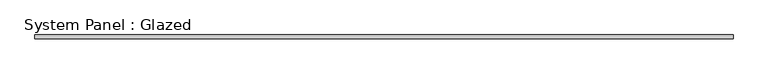
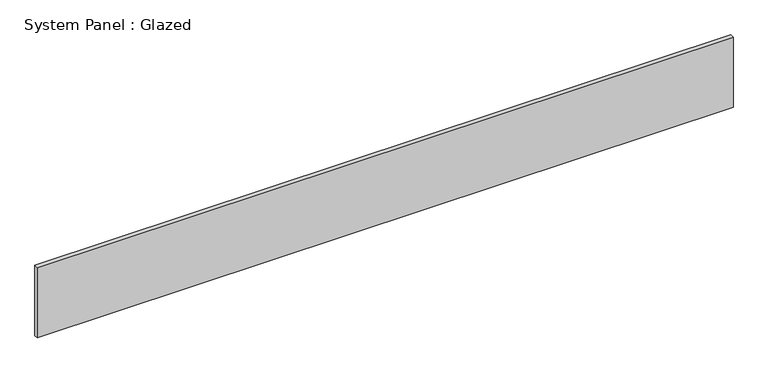
"""IFC4 building model written with IfcOpenShell, lengths in millimetres: plate geometry, System Panel : Glazed."""

from ifc_helpers import new_model, si_unit, origin, origin_with_axes, place, context, project, spatial, polyline, outline, extrude, source, transform, mapped, element, save


def system_panel_glazed_6f34b03a(model_context):
    return source(origin(), model_context, "Body", "SweptSolid", [
        extrude(outline(polyline([(2324.1, 19.05), (-2324.1, 19.05), (-2324.1, 44.45), (2324.1, 44.45), (2324.1, 19.05)])), origin_with_axes(), (0.0, 0.0, 1.0), 495.3),
    ])


if __name__ == "__main__":
    model = new_model("IFC4")
    model_context = context("Model", 3, world=origin())
    ifc_project = project(units=[si_unit("LENGTHUNIT", "METRE", prefix="MILLI")], contexts=[model_context])
    site = spatial("IfcSite", under=ifc_project)
    building = spatial("IfcBuilding", under=site)
    placement = place(None, origin())
    system_panel_glazed_shape = system_panel_glazed_6f34b03a(model_context)
    element("IfcPlate", 1, ObjectType="System Panel : Glazed", at=placement, inside=building, context=model_context, shape_type="MappedRepresentation", body=[
        mapped(system_panel_glazed_shape, transform((0.0, 0.0, 0.0), x_axis=(1.0, 0.0, 0.0), y_axis=(0.0, 1.0, 0.0), z_axis=(0.0, 0.0, 1.0))),
    ])
    save(model, "model.ifc")

# Revit data of these elements
# Type "System Panel : Glazed"
#   Construction Type Id = "GSP4R"
#   Analytic Construction = "1/8 in Pilkington single glazing"
#   Visual Light Transmittance = 0.9
#   Solar Heat Gain Coefficient = 0.86
#   Heat Transfer Coefficient (U) = 1.18115 BTU/(h·ft²·°F)
#   Define Thermal Properties by = 1
# Element 1 (IfcPlate, "System Panel : Glazed")
#   Materials on its faces: "Glass"
# Materials
#   "Glass": class "Glass", colour RGB 0 128 192, transparency 0.75, Description = "Soda Lime Glass", Cost = 0
